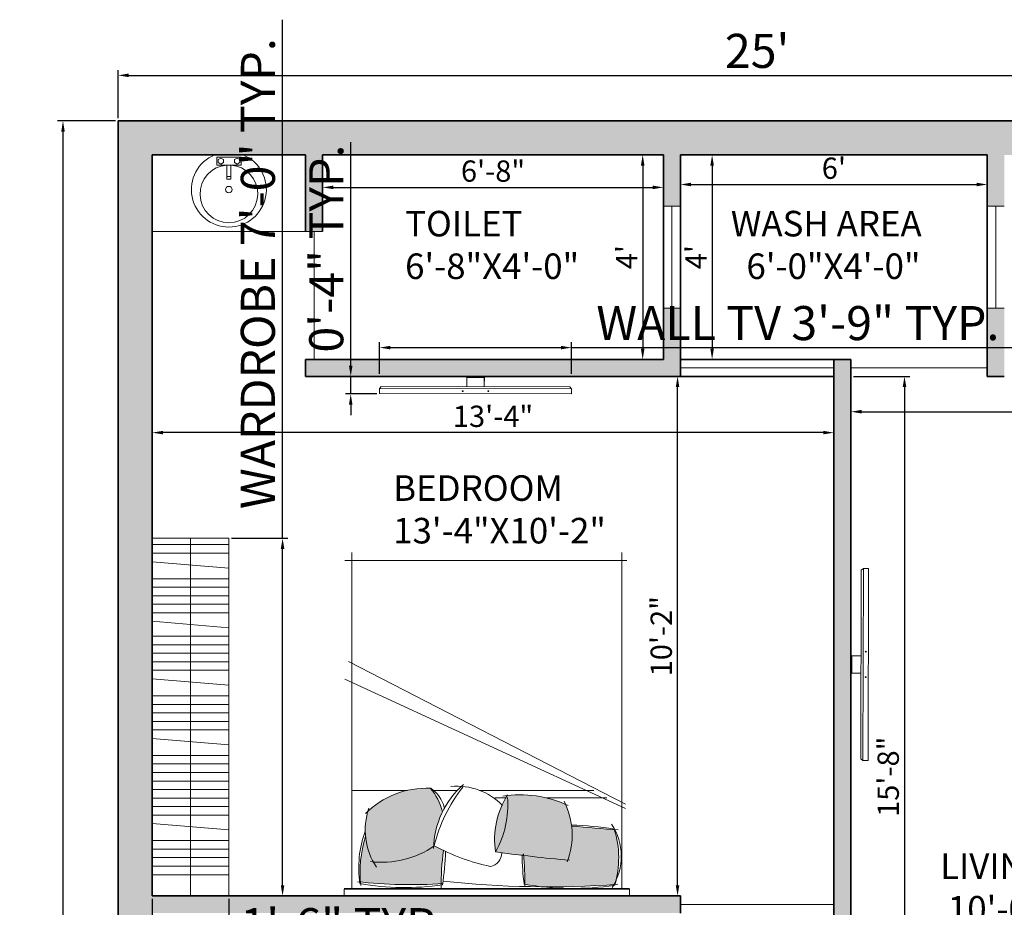
# Model space of a CAD drawing. Units: inches. Extents: x 3259 to 4981, y 1402 to 2026.
# Tile 3 of 11: x 3278 to 3509, y 1722 to 1931. Entities that reach past the tile are written whole.
import ezdxf

# ---------------------------------------------------------------- set-up
doc = ezdxf.new("R2010")
doc.units = ezdxf.units.IN
for name, color, linetype, lineweight in [('0.10', 252, 'Continuous', 9), ('A-ANNO-DIMS', 2, 'Continuous', 13), ('A-AREA-IDEN', 7, 'Continuous', 18), ('A-DOOR', 3, 'Continuous', 18), ('A-EQPM', 8, 'Continuous', 18), ('A-FLOR-CASE', 8, 'Continuous', 18), ('A-FLOR-FIXT', 9, 'Continuous', 18), ('A-FURN', 8, 'Continuous', 13), ('A-GLAZ', 4, 'Continuous', 18), ('A-WALL', 7, 'Continuous', 35), ('A-WALL-PATT', 252, 'Continuous', 13)]:
    doc.layers.add(name, color=color, linetype=linetype, lineweight=lineweight)
doc.layers.add('A-FURN-PATT', color=116, linetype='Continuous', lineweight=13, true_color=0x136734)
doc.styles.get("Standard").update_dxf_attribs({"font": 'arial.ttf'})
doc.dimstyles.new('ISO-25', dxfattribs={"dimtxt": 8, "dimasz": 2.5, "dimexe": 1.25, "dimexo": 0.625, "dimtad": 1, "dimdec": 1, "dimlunit": 3, "dimtxsty": 'Standard', "dimcen": 2.5, "dimclrd": 4, "dimclre": 4, "dimclrt": 1, "dimadec": 0, "dimazin": 0, "dimtfac": 1, "dimtdec": 1, "dimtmove": 0, "dimatfit": 3, "dimfxl": 1, "dimarcsym": 0})

# ---------------------------------------------------------------- blocks, each defined once
blk = doc.blocks.new('camita')
at = {"layer": '0.10'}
for p, q in [((-0.85, -0.045), (0.85, -0.045)), ((-0.805, -0.045), (-0.805, -2.0485)), ((0.805, -0.045), (0.805, -2.0485)), ((-0.8271, -0.521), (0.8464, -1.2932)), ((-0.8271, -0.5476), (0.8236, -1.3992)), ((-0.7161, -0.585), (-0.3554, -0.585)), ((-0.1136, -0.585), (-0.0485, -0.585)), ((-0.638, -0.63), (0.0434, -0.63)), ((0.1749, -0.63), (0.3179, -0.63)), ((0.4739, -0.63), (0.805, -0.63)), ((-0.8354, -2), (0.8464, -2))]:
    blk.add_line(p, q, dxfattribs=at)
blk.add_lwpolyline([(-0.85, -0.0405), (0.85, -0.0405), (0.85, 0), (-0.85, 0)], close=True, dxfattribs=at)
for centre, radius, start, end in [((-0.4574, -0.2364), 0.3443, 147.50996, 213.83359), ((-0.3639, -5.8457), 5.7909, 83.80731, 94.12107), ((-0.5104, -1.7232), 1.6781, 80.12554, 98.66187), ((2.3534, -0.0532), 2.5803, 180.10628, 184.38541), ((-1.4396, -0.0609), 1.7117, 352.92911, 0.39592), ((0.4863, -1.6286), 1.5781, 80.16015, 98.05996), ((-0.1997, -0.2266), 0.5864, 163.92635, 197.14087), ((-1.5443, -0.2452), 1.3333, 359.93941, 7.55329), ((1.5815, -0.2893), 1.3353, 170.38021, 178.99138), ((0.4524, -3.0675), 2.9996, 83.90257, 93.67595), ((0.0294, -0.1377), 0.7262, 342.58415, 6.00484), ((0.1326, -0.1696), 0.6307, 339.92303, 8.74334), ((0.3203, -0.3944), 0.4043, 341.45245, 33.45121), ((-0.0543, -0.3633), 0.4542, 159.30257, 206.50263), ((-1.3301, -9.6748), 9.4985, 82.27078, 84.93989), ((-0.007, -0.258), 0.0828, 100.01798, 179.73597), ((-0.2931, -1.4378), 1.2903, 61.97485, 77.84351), ((0.6265, -0.7518), 0.5508, 82.96906, 124.67388), ((0.4585, -0.5454), 0.5842, 151.04555, 184.14969), ((-0.5341, -0.3393), 0.4875, 327.26442, 9.0473), ((-0.1986, -0.2742), 0.5159, 310.73945, 359.05759), ((-0.5673, -0.0868), 0.9057, 321.69527, 346.46261), ((-1.8672, -14.986), 14.6323, 84.65974, 85.75157), ((-0.4598, 1.4861), 1.9092, 260.95299, 268.65169), ((0.5707, -0.4317), 0.3145, 192.93877, 221.96363), ((0.3612, -0.133), 0.5096, 267.25889, 315.29965), ((-0.2002, 0.064), 0.6673, 244.78094, 279.06058), ((0.179, -0.272), 0.3828, 224.52836, 275.22287), ((0.4384, -0.4834), 0.1898, 193.68485, 236.70352)]:
    blk.add_arc(centre, radius, start, end, dxfattribs=at)
blk = doc.blocks.new('M_BATH_BASIN_Basin - Oval_P')
at = {"color": 0, "linetype": 'ByBlock', "lineweight": -2}
blk.add_lwpolyline([(0, 89.5, -5.027337), (0, -89.5)], format="xyb", close=True, dxfattribs=at)
blk.add_lwpolyline([(63.2, 12, -30), (63.2, -12, -1.097889)], format="xyb", dxfattribs=at)
for points in [[(13.2, -76.2), (13.2, 76.2), (63.2, 76.2), (63.2, -76.2)], [(19.1, 50.8), (28.7, 67.3), (47.7, 67.3), (57.2, 50.8), (47.7, 34.3), (28.7, 34.3)]]:
    blk.add_lwpolyline(points, close=True, dxfattribs=at)
for points in [[(63.2, 12), (151.6, 12), (151.6, -12), (63.2, -12)], [(134.3, 12), (134.3, -12)], [(28.7, -34.3), (47.7, -34.3), (57.2, -50.8), (47.7, -67.3), (28.7, -67.3), (19.1, -50.8), (28.7, -34.3)]]:
    blk.add_lwpolyline(points, dxfattribs=at)
blk.add_circle((216.2, 0), 20.1, dxfattribs=at)
at = {"layer": 'Defpoints'}
for p in [(0, 234), (0, -234)]:
    blk.add_point(p, dxfattribs=at)
blk = doc.blocks.new('*D21')
at = {"layer": 'A-ANNO-DIMS', "color": 0, "lineweight": -2, "transparency": 16777216}
for p, q in [((3301.16, 1907.74), (3301.16, 1919.06)), ((3601.16, 1907.74), (3601.16, 1919.06)), ((3303.66, 1917.81), (3598.66, 1917.81))]:
    blk.add_line(p, q, dxfattribs=at)
at = {"layer": 'A-ANNO-DIMS', "color": 0, "transparency": 16777216}
for points in [[(3303.66, 1918.23), (3303.66, 1917.39), (3301.16, 1917.81)], [(3598.66, 1918.23), (3598.66, 1917.39), (3601.16, 1917.81)]]:
    blk.add_solid(points, dxfattribs=at)
at = {"layer": 'Defpoints', "color": 0, "transparency": 16777216}
for p in [(3601.16, 1917.81), (3301.16, 1907.12), (3601.16, 1907.12)]:
    blk.add_point(p, dxfattribs=at)
at = {"layer": 'A-ANNO-DIMS', "color": 0, "transparency": 16777216, "insert": (3451.16, 1922.52), "char_height": 8, "attachment_point": 5}
blk.add_mtext("25'", dxfattribs=at)
blk = doc.blocks.new('*D22')
at = {"layer": 'A-ANNO-DIMS', "color": 0, "lineweight": -2, "transparency": 16777216}
for p, q in [((3300.54, 1907.12), (3286.97, 1907.12)), ((3288.22, 1904.62), (3288.22, 1477.62)), ((3300.54, 1475.12), (3286.97, 1475.12))]:
    blk.add_line(p, q, dxfattribs=at)
at = {"layer": 'A-ANNO-DIMS', "color": 0, "transparency": 16777216}
for points in [[(3287.81, 1904.62), (3288.64, 1904.62), (3288.22, 1907.12)], [(3287.81, 1477.62), (3288.64, 1477.62), (3288.22, 1475.12)]]:
    blk.add_solid(points, dxfattribs=at)
at = {"layer": 'Defpoints', "color": 0, "transparency": 16777216}
for p in [(3301.16, 1907.12), (3288.22, 1475.12), (3301.16, 1475.12)]:
    blk.add_point(p, dxfattribs=at)
at = {"layer": 'A-ANNO-DIMS', "color": 0, "transparency": 16777216, "insert": (3283.51, 1691.12), "char_height": 8, "attachment_point": 5, "rotation": 90}
blk.add_mtext("36'", dxfattribs=at)
blk = doc.blocks.new('*D23')
at = {"layer": 'A-ANNO-DIMS', "color": 0, "lineweight": -2, "transparency": 16777216}
for p, q in [((3309.16, 1846.49), (3309.16, 1832.67)), ((3469.16, 1846.49), (3469.16, 1832.67)), ((3466.66, 1833.92), (3311.66, 1833.92))]:
    blk.add_line(p, q, dxfattribs=at)
at = {"layer": 'A-ANNO-DIMS', "color": 0, "transparency": 16777216}
for points in [[(3311.66, 1834.34), (3311.66, 1833.51), (3309.16, 1833.92)], [(3466.66, 1834.34), (3466.66, 1833.51), (3469.16, 1833.92)]]:
    blk.add_solid(points, dxfattribs=at)
at = {"layer": 'Defpoints', "color": 0, "transparency": 16777216}
for p in [(3309.16, 1847.12), (3469.16, 1847.12), (3309.16, 1833.92)]:
    blk.add_point(p, dxfattribs=at)
at = {"layer": 'A-ANNO-DIMS', "color": 0, "transparency": 16777216, "insert": (3389.16, 1837.1), "char_height": 5, "attachment_point": 5}
blk.add_mtext('13\'-4"', dxfattribs=at)
blk = doc.blocks.new('*D24')
at = {"layer": 'A-ANNO-DIMS', "color": 0, "lineweight": -2, "transparency": 16777216}
for p, q in [((3432.54, 1847.12), (3431.22, 1847.12)), ((3432.47, 1727.62), (3432.47, 1844.62)), ((3432.54, 1725.12), (3431.22, 1725.12))]:
    blk.add_line(p, q, dxfattribs=at)
at = {"layer": 'A-ANNO-DIMS', "color": 0, "transparency": 16777216}
for points in [[(3432.05, 1844.62), (3432.89, 1844.62), (3432.47, 1847.12)], [(3432.05, 1727.62), (3432.89, 1727.62), (3432.47, 1725.12)]]:
    blk.add_solid(points, dxfattribs=at)
at = {"layer": 'Defpoints', "color": 0, "transparency": 16777216}
for p in [(3432.47, 1847.12), (3433.16, 1847.12), (3433.16, 1725.12)]:
    blk.add_point(p, dxfattribs=at)
at = {"layer": 'A-ANNO-DIMS', "color": 0, "transparency": 16777216, "insert": (3429.29, 1786.12), "char_height": 5, "attachment_point": 5, "rotation": 90}
blk.add_mtext('10\'-2"', dxfattribs=at)
blk = doc.blocks.new('*D25')
at = {"layer": 'A-ANNO-DIMS', "color": 0, "lineweight": -2, "transparency": 16777216}
for p, q in [((3593.16, 1846.49), (3593.16, 1837.58)), ((3473.16, 1843.37), (3473.16, 1837.58)), ((3475.66, 1838.83), (3590.66, 1838.83))]:
    blk.add_line(p, q, dxfattribs=at)
at = {"layer": 'A-ANNO-DIMS', "color": 0, "transparency": 16777216}
for points in [[(3475.66, 1839.25), (3475.66, 1838.42), (3473.16, 1838.83)], [(3590.66, 1839.25), (3590.66, 1838.42), (3593.16, 1838.83)]]:
    blk.add_solid(points, dxfattribs=at)
at = {"layer": 'Defpoints', "color": 0, "transparency": 16777216}
for p in [(3593.16, 1847.12), (3473.16, 1844), (3593.16, 1838.83)]:
    blk.add_point(p, dxfattribs=at)
at = {"layer": 'A-ANNO-DIMS', "color": 0, "transparency": 16777216, "insert": (3533.16, 1842.01), "char_height": 5, "attachment_point": 5}
blk.add_mtext("10'", dxfattribs=at)
blk = doc.blocks.new('*D26')
at = {"layer": 'A-ANNO-DIMS', "color": 0, "lineweight": -2, "transparency": 16777216}
for p, q in [((3473.79, 1847.12), (3486.99, 1847.12)), ((3485.74, 1844.62), (3485.74, 1661.62)), ((3473.79, 1659.12), (3486.99, 1659.12))]:
    blk.add_line(p, q, dxfattribs=at)
at = {"layer": 'A-ANNO-DIMS', "color": 0, "transparency": 16777216}
for points in [[(3485.32, 1844.62), (3486.16, 1844.62), (3485.74, 1847.12)], [(3485.32, 1661.62), (3486.16, 1661.62), (3485.74, 1659.12)]]:
    blk.add_solid(points, dxfattribs=at)
at = {"layer": 'Defpoints', "color": 0, "transparency": 16777216}
for p in [(3473.16, 1847.12), (3473.16, 1659.12), (3485.74, 1659.12)]:
    blk.add_point(p, dxfattribs=at)
at = {"layer": 'A-ANNO-DIMS', "color": 0, "transparency": 16777216, "insert": (3482.56, 1753.12), "char_height": 5, "attachment_point": 5, "rotation": 90}
blk.add_mtext('15\'-8"', dxfattribs=at)
blk = doc.blocks.new('*D35')
at = {"layer": 'A-ANNO-DIMS', "color": 0, "lineweight": -2, "transparency": 16777216}
for p, q in [((3349.16, 1898.49), (3349.16, 1890.25)), ((3429.16, 1898.49), (3429.16, 1890.25)), ((3351.66, 1891.5), (3426.66, 1891.5))]:
    blk.add_line(p, q, dxfattribs=at)
at = {"layer": 'A-ANNO-DIMS', "color": 0, "transparency": 16777216}
for points in [[(3351.66, 1891.92), (3351.66, 1891.09), (3349.16, 1891.5)], [(3426.66, 1891.92), (3426.66, 1891.09), (3429.16, 1891.5)]]:
    blk.add_solid(points, dxfattribs=at)
at = {"layer": 'Defpoints', "color": 0, "transparency": 16777216}
for p in [(3349.16, 1899.12), (3429.16, 1899.12), (3429.16, 1891.5)]:
    blk.add_point(p, dxfattribs=at)
at = {"layer": 'A-ANNO-DIMS', "color": 0, "transparency": 16777216, "insert": (3389.16, 1894.68), "char_height": 5, "attachment_point": 5}
blk.add_mtext('6\'-8"', dxfattribs=at)
blk = doc.blocks.new('*D36')
at = {"layer": 'A-ANNO-DIMS', "color": 0, "lineweight": -2, "transparency": 16777216}
for p, q in [((3428.54, 1899.12), (3423.04, 1899.12)), ((3424.29, 1896.62), (3424.29, 1853.62)), ((3428.54, 1851.12), (3423.04, 1851.12))]:
    blk.add_line(p, q, dxfattribs=at)
at = {"layer": 'A-ANNO-DIMS', "color": 0, "transparency": 16777216}
for points in [[(3423.87, 1896.62), (3424.71, 1896.62), (3424.29, 1899.12)], [(3423.87, 1853.62), (3424.71, 1853.62), (3424.29, 1851.12)]]:
    blk.add_solid(points, dxfattribs=at)
at = {"layer": 'Defpoints', "color": 0, "transparency": 16777216}
for p in [(3429.16, 1899.12), (3424.29, 1851.12), (3429.16, 1851.12)]:
    blk.add_point(p, dxfattribs=at)
at = {"layer": 'A-ANNO-DIMS', "color": 0, "transparency": 16777216, "insert": (3421.17, 1875.12), "char_height": 5, "attachment_point": 5, "rotation": 90}
blk.add_mtext("4'", dxfattribs=at)
blk = doc.blocks.new('*D37')
at = {"layer": 'A-ANNO-DIMS', "color": 0, "lineweight": -2, "transparency": 16777216}
for p, q in [((3433.16, 1898.49), (3433.16, 1890.93)), ((3505.16, 1898.49), (3505.16, 1890.93)), ((3435.66, 1892.18), (3502.66, 1892.18))]:
    blk.add_line(p, q, dxfattribs=at)
at = {"layer": 'A-ANNO-DIMS', "color": 0, "transparency": 16777216}
for points in [[(3435.66, 1892.6), (3435.66, 1891.76), (3433.16, 1892.18)], [(3502.66, 1892.6), (3502.66, 1891.76), (3505.16, 1892.18)]]:
    blk.add_solid(points, dxfattribs=at)
at = {"layer": 'Defpoints', "color": 0, "transparency": 16777216}
for p in [(3433.16, 1899.12), (3505.16, 1899.12), (3505.16, 1892.18)]:
    blk.add_point(p, dxfattribs=at)
at = {"layer": 'A-ANNO-DIMS', "color": 0, "transparency": 16777216, "insert": (3469.16, 1895.36), "char_height": 5, "attachment_point": 5}
blk.add_mtext("6'", dxfattribs=at)
blk = doc.blocks.new('*D38')
at = {"layer": 'A-ANNO-DIMS', "color": 0, "lineweight": -2, "transparency": 16777216}
for p, q in [((3433.79, 1899.12), (3441.83, 1899.12)), ((3440.58, 1896.62), (3440.58, 1853.62)), ((3433.79, 1851.12), (3441.83, 1851.12))]:
    blk.add_line(p, q, dxfattribs=at)
at = {"layer": 'A-ANNO-DIMS', "color": 0, "transparency": 16777216}
for points in [[(3440.16, 1896.62), (3441, 1896.62), (3440.58, 1899.12)], [(3440.16, 1853.62), (3441, 1853.62), (3440.58, 1851.12)]]:
    blk.add_solid(points, dxfattribs=at)
at = {"layer": 'Defpoints', "color": 0, "transparency": 16777216}
for p in [(3433.16, 1899.12), (3433.16, 1851.12), (3440.58, 1851.12)]:
    blk.add_point(p, dxfattribs=at)
at = {"layer": 'A-ANNO-DIMS', "color": 0, "transparency": 16777216, "insert": (3437.45, 1875.12), "char_height": 5, "attachment_point": 5, "rotation": 90}
blk.add_mtext("4'", dxfattribs=at)
blk = doc.blocks.new('WARDROBE-84IN')
for p, q in [((0, 84), (18, 84)), ((9, 0), (9, 84)), ((18, 0), (18, 84)), ((18, 82.5), (0, 82.5)), ((18, 80.5), (0, 80.5)), ((18, 77), (0, 78.5)), ((18, 74.5), (0, 74.5)), ((18, 72.5), (0, 72.5)), ((18, 70.5), (0, 70.5)), ((18, 68.5), (0, 68.5)), ((18, 66.5), (0, 66.5)), ((18, 63), (0, 64.5)), ((18, 61), (0, 61)), ((18, 59), (0, 59)), ((18, 57), (0, 57)), ((18, 55), (0, 55)), ((18, 53), (0, 53)), ((18, 49.5), (0, 51)), ((18, 47), (0, 47)), ((18, 45), (0, 45)), ((18, 43), (0, 43)), ((18, 41), (0, 41)), ((18, 39), (0, 39)), ((18, 35.5), (0, 37)), ((18, 33), (0, 33)), ((18, 31), (0, 31)), ((18, 29), (0, 29)), ((18, 27), (0, 27)), ((18, 25), (0, 25)), ((18, 23), (0, 23)), ((18, 21), (0, 21)), ((18, 19), (0, 19)), ((18, 15.5), (0, 17)), ((18, 13), (0, 13)), ((18, 11), (0, 11)), ((18, 9), (0, 9)), ((18, 7), (0, 7)), ((18, 5), (0, 5))]:
    blk.add_line(p, q)
blk = doc.blocks.new('TV-WALL-MOUNT')
for p, q in [((20.48, 4.12), (20.47, 1.73)), ((20.48, 4.12), (20.52, 4.12)), ((20.52, 4.12), (20.52, 1.73)), ((20.52, 3.88), (24.55, 3.88)), ((24.55, 4.12), (24.55, 1.72)), ((24.55, 4.12), (24.6, 4.12)), ((24.6, 4.12), (24.59, 1.72)), ((0, 1.29), (0.41, 1.77)), ((0.41, 1.77), (44.66, 1.68)), ((45.06, 1.2), (44.66, 1.68))]:
    blk.add_line(p, q)
blk.add_lwpolyline([(0, 0.09), (45.06, 0), (45.06, 1.2), (0, 1.29), (0, 0.09)])
for centre in [(19.53, 0.65), (25.53, 0.64)]:
    blk.add_circle(centre, 0.0959)
blk = doc.blocks.new('VENT-24x4')
for p, q in [((0, 24), (4, 24)), ((2, 24), (2, 0)), ((0, 0), (4, 0))]:
    blk.add_line(p, q)
blk = doc.blocks.new('*D164')
at = {"layer": 'A-ANNO-DIMS', "color": 4, "lineweight": -2, "transparency": 16777216}
for p, q in [((3339.76, 1809.12), (3339.76, 1930.88)), ((3327.79, 1809.12), (3341.01, 1809.12)), ((3339.76, 1727.62), (3339.76, 1806.62)), ((3327.79, 1725.12), (3341.01, 1725.12))]:
    blk.add_line(p, q, dxfattribs=at)
at = {"layer": 'A-ANNO-DIMS', "color": 4, "transparency": 16777216}
for points in [[(3339.35, 1806.62), (3340.18, 1806.62), (3339.76, 1809.12)], [(3339.35, 1727.62), (3340.18, 1727.62), (3339.76, 1725.12)]]:
    blk.add_solid(points, dxfattribs=at)
at = {"layer": 'Defpoints', "color": 0, "transparency": 16777216}
for p in [(3327.16, 1809.12), (3339.76, 1809.12), (3327.16, 1725.12)]:
    blk.add_point(p, dxfattribs=at)
at = {"layer": 'A-ANNO-DIMS', "color": 1, "transparency": 16777216, "insert": (3335, 1871.25), "char_height": 8, "attachment_point": 5, "rotation": 90}
blk.add_mtext('WARDROBE 7\'-0" TYP.', dxfattribs=at)
blk = doc.blocks.new('*D165')
at = {"layer": 'A-ANNO-DIMS', "color": 4, "lineweight": -2, "transparency": 16777216}
for p, q in [((3309.16, 1724.49), (3309.16, 1711.27)), ((3327.16, 1724.49), (3327.16, 1711.27)), ((3311.66, 1712.52), (3324.66, 1712.52)), ((3327.16, 1712.52), (3378.93, 1712.52))]:
    blk.add_line(p, q, dxfattribs=at)
at = {"layer": 'A-ANNO-DIMS', "color": 4, "transparency": 16777216}
for points in [[(3311.66, 1712.93), (3311.66, 1712.1), (3309.16, 1712.52)], [(3324.66, 1712.93), (3324.66, 1712.1), (3327.16, 1712.52)]]:
    blk.add_solid(points, dxfattribs=at)
at = {"layer": 'Defpoints', "color": 0, "transparency": 16777216}
for p in [(3309.16, 1725.12), (3327.16, 1725.12), (3327.16, 1712.52)]:
    blk.add_point(p, dxfattribs=at)
at = {"layer": 'A-ANNO-DIMS', "color": 1, "transparency": 16777216, "insert": (3354.29, 1717.23), "char_height": 8, "attachment_point": 5}
blk.add_mtext('1\'-6" TYP.', dxfattribs=at)
blk = doc.blocks.new('*D168')
at = {"layer": 'A-ANNO-DIMS', "color": 4, "lineweight": -2, "transparency": 16777216}
for p, q in [((3362.52, 1847.75), (3362.52, 1855.13)), ((3365.02, 1853.88), (3405.08, 1853.88)), ((3407.58, 1847.75), (3407.58, 1855.13)), ((3407.58, 1853.88), (3511.34, 1853.88))]:
    blk.add_line(p, q, dxfattribs=at)
at = {"layer": 'A-ANNO-DIMS', "color": 4, "transparency": 16777216}
for points in [[(3365.02, 1854.3), (3365.02, 1853.47), (3362.52, 1853.88)], [(3405.08, 1854.3), (3405.08, 1853.47), (3407.58, 1853.88)]]:
    blk.add_solid(points, dxfattribs=at)
at = {"layer": 'Defpoints', "color": 0, "transparency": 16777216}
for p in [(3407.58, 1853.88), (3362.52, 1847.13), (3407.58, 1847.13)]:
    blk.add_point(p, dxfattribs=at)
at = {"layer": 'A-ANNO-DIMS', "color": 1, "transparency": 16777216, "insert": (3460.71, 1858.6), "char_height": 8, "attachment_point": 5}
blk.add_mtext('WALL TV 3\'-9" TYP.', dxfattribs=at)
blk = doc.blocks.new('*D169')
at = {"layer": 'A-ANNO-DIMS', "color": 4, "lineweight": -2, "transparency": 16777216}
for p, q in [((3355.76, 1849.63), (3355.76, 1902.14)), ((3361.89, 1847.13), (3354.51, 1847.13)), ((3355.76, 1843), (3355.76, 1847.13)), ((3361.89, 1843), (3354.51, 1843)), ((3355.76, 1840.5), (3355.76, 1838))]:
    blk.add_line(p, q, dxfattribs=at)
at = {"layer": 'A-ANNO-DIMS', "color": 4, "transparency": 16777216}
for points in [[(3355.34, 1849.63), (3356.17, 1849.63), (3355.76, 1847.13)], [(3355.34, 1840.5), (3356.17, 1840.5), (3355.76, 1843)]]:
    blk.add_solid(points, dxfattribs=at)
at = {"layer": 'Defpoints', "color": 0, "transparency": 16777216}
for p in [(3355.76, 1847.13), (3362.52, 1847.13), (3362.52, 1843)]:
    blk.add_point(p, dxfattribs=at)
at = {"layer": 'A-ANNO-DIMS', "color": 1, "transparency": 16777216, "insert": (3351.05, 1877.13), "char_height": 8, "attachment_point": 5, "rotation": 90}
blk.add_mtext('0\'-4" TYP.', dxfattribs=at)

msp = doc.modelspace()

# ---------------------------------------------------------------- hatches: boundary and pattern name
at = {"layer": 'A-FURN-PATT'}
h = msp.add_hatch(color=256, dxfattribs=at)
h.dxf.hatch_style = 1
h.paths.add_polyline_path([(3392.47, 1748.69, 0.181694), (3389.77, 1735.46, 0.011408), (3406.73, 1733.55, 0.189536), (3406.2, 1746.63, 0.134508)])
h.paths.add_polyline_path([(3375.22, 1736.79, -0.104045), (3377.29, 1744.89, 0.127326), (3374.43, 1750.4, 0.202559), (3359.77, 1745.01, 0.194952), (3361.05, 1733.12, 0.173835)])
h = msp.add_hatch(color=256, dxfattribs=at)
h.dxf.hatch_style = 1
h.paths.add_polyline_path([(3407.59, 1741.55, -0.113891), (3406.73, 1733.55, -0.006967), (3396.36, 1734.62, -0.016701), (3396.63, 1727.84, 0.015442), (3400.67, 1727.28, 0.01851), (3417.54, 1727.8, 0.020657), (3418.04, 1728.8, 0.131047), (3417.67, 1740.69, -0.004387)])
h.paths.add_polyline_path([(3377.5, 1735.81, -0.011742), (3375.36, 1736.88, -0.175864), (3361.05, 1733.12, -0.098488), (3359.24, 1739.06, 0.094792), (3358.02, 1728.39, 0.040212), (3376.99, 1728, -0.029051)])
at = {"layer": 'A-WALL-PATT'}
h = msp.add_hatch(color=256, dxfattribs=at)
h.dxf.hatch_style = 1
h.paths.add_polyline_path([(3601.16, 1907.12), (3301.16, 1907.12), (3301.16, 1475.12), (3398.16, 1475.12), (3398.16, 1483.12), (3309.16, 1483.12), (3309.16, 1579.12), (3421.16, 1579.12), (3421.16, 1583.12), (3309.16, 1583.12), (3309.16, 1721.12), (3433.16, 1721.12), (3433.16, 1725.12), (3309.16, 1725.12), (3309.16, 1899.12), (3345.16, 1899.12), (3345.16, 1881.12), (3349.16, 1881.12), (3349.16, 1899.12), (3429.16, 1899.12), (3429.16, 1887.12), (3433.16, 1887.12), (3433.16, 1899.12), (3505.16, 1899.12), (3505.16, 1887.12), (3509.16, 1887.12), (3509.16, 1899.12), (3593.16, 1899.12), (3593.16, 1851.12), (3539.16, 1851.12), (3539.16, 1847.12), (3593.16, 1847.12), (3593.16, 1659.12), (3587.16, 1659.12), (3587.16, 1651.12), (3593.16, 1651.12), (3593.16, 1475.12), (3601.16, 1475.12)])
h.paths.add_polyline_path([(3433.16, 1863.12), (3429.16, 1863.12), (3429.16, 1851.12), (3345.16, 1851.12), (3345.16, 1847.12), (3382.99, 1847.12), (3382.99, 1847.13), (3383.04, 1847.13), (3383.04, 1847.12), (3387.07, 1847.12), (3387.07, 1847.12), (3387.11, 1847.12), (3433.16, 1847.12)], flags=17)
h.paths.add_polyline_path([(3509.16, 1863.12), (3505.16, 1863.12), (3505.16, 1847.12), (3509.16, 1847.12)], flags=17)
h.paths.add_polyline_path([(3473.16, 1851.12), (3469.16, 1851.12), (3469.16, 1715.12), (3473.16, 1715.12), (3473.16, 1777.43), (3473.16, 1777.43), (3473.16, 1777.47), (3473.16, 1777.47), (3473.16, 1781.5), (3473.16, 1781.5), (3473.16, 1781.55)], flags=17)
h.paths.add_polyline_path([(3491.16, 1659.12), (3473.16, 1659.12), (3473.16, 1667.12), (3469.16, 1667.12), (3469.16, 1483.12), (3473.16, 1483.12), (3473.16, 1651.12), (3491.16, 1651.12)], flags=17)
h.paths.add_polyline_path([(3551.16, 1659.12), (3539.16, 1659.12), (3539.16, 1651.12), (3551.16, 1651.12)], flags=17)
h.paths.add_polyline_path([(3473.16, 1483.12), (3458.16, 1483.12), (3458.16, 1475.12), (3473.16, 1475.12)], flags=17)

# ---------------------------------------------------------------- linework, layer by layer
at = {"layer": 'A-DOOR'}
for p, q in [((3347.16, 1881.12), (3347.16, 1851.12)), ((3473.16, 1849.12), (3505.16, 1849.12)), ((3433.16, 1723.12), (3469.16, 1723.12))]:
    msp.add_line(p, q, dxfattribs=at)
at = {"layer": 'A-FLOR-CASE'}
msp.add_line((3309.16, 1881.12), (3349.16, 1881.12), dxfattribs=at)
at = {"layer": 'A-GLAZ'}
msp.add_line((3433.16, 1849.12), (3469.16, 1849.12), dxfattribs=at)
at = {"layer": 'A-WALL'}
for p, q in [((3309.16, 1899.12), (3345.16, 1899.12)), ((3309.16, 1725.12), (3309.16, 1899.12)), ((3345.16, 1899.12), (3345.16, 1881.12)), ((3349.16, 1899.12), (3349.16, 1881.12)), ((3349.16, 1899.12), (3429.16, 1899.12)), ((3429.16, 1899.12), (3429.16, 1851.12)), ((3433.16, 1899.12), (3433.16, 1847.12)), ((3433.16, 1899.12), (3505.16, 1899.12)), ((3505.16, 1899.12), (3505.16, 1847.12)), ((3345.16, 1851.12), (3429.16, 1851.12)), ((3345.16, 1851.12), (3345.16, 1847.12)), ((3433.16, 1851.12), (3473.16, 1851.12)), ((3469.16, 1715.12), (3469.16, 1851.12)), ((3473.16, 1715.12), (3473.16, 1851.12)), ((3345.16, 1847.12), (3469.16, 1847.12)), ((3505.16, 1847.12), (3509.16, 1847.12)), ((3309.16, 1725.12), (3433.16, 1725.12)), ((3433.16, 1721.12), (3433.16, 1725.12))]:
    msp.add_line(p, q, dxfattribs=at)
msp.add_lwpolyline([(3473.16, 1475.12), (3301.16, 1475.12), (3301.16, 1907.12), (3601.16, 1907.12), (3601.16, 1475.12), (3593.16, 1475.12)], dxfattribs=at)

# ---------------------------------------------------------------- block references
at = {"layer": 'A-EQPM'}
msp.add_blockref('TV-WALL-MOUNT', (3362.52, 1843), dxfattribs=at)
at = {"layer": 'A-EQPM', "rotation": 90}
msp.add_blockref('TV-WALL-MOUNT', (3477.28, 1756.95), dxfattribs=at)
at = {"layer": 'A-FLOR-CASE'}
msp.add_blockref('WARDROBE-84IN', (3309.16, 1725.12), dxfattribs=at)
at = {"layer": 'A-FLOR-FIXT', "xscale": -0.0376189459335944, "yscale": 0.0376189459335944, "zscale": 0.0376189459335944, "rotation": 90}
msp.add_blockref('M_BATH_BASIN_Basin - Oval_P', (3327.16, 1899.12), dxfattribs=at)
at = {"layer": 'A-FURN', "xscale": 39.375, "yscale": 39.375, "zscale": 39.375, "rotation": 180}
msp.add_blockref('camita', (3387.7, 1725.12), dxfattribs=at)
at = {"layer": 'A-GLAZ'}
msp.add_blockref('VENT-24x4', (3429.16, 1863.12), dxfattribs=at)
at = {"layer": 'A-GLAZ', "rotation": 180}
msp.add_blockref('VENT-24x4', (3509.16, 1887.12), dxfattribs=at)

# ---------------------------------------------------------------- texts
at = {"layer": 'A-AREA-IDEN', "char_height": 6, "attachment_point": 1}
for s, width, insert in [('TOILET\\P6\'-8"X4\'-0"', 127.3061, (3368.52, 1885.99)), ('WASH AREA\\P  6\'-0"X4\'-0"', 127.3061, (3444.97, 1885.99)), ('BEDROOM\\P13\'-4"X10\'-2"', 86.9528, (3365.72, 1823.9)), ('LIVING ROOM\\P 10\'-0"X15\'-8"', 127.3061, (3494.1, 1735.12))]:
    msp.add_mtext_dynamic_manual_height_columns(s, width=width, gutter_width=12.5, heights=[0], dxfattribs=dict(at, insert=insert))

# ---------------------------------------------------------------- dimensions: what is measured, and where the dimension line sits
at = {"layer": 'A-ANNO-DIMS'}
for base, p1, p2, text, picture, middle in [((3339.76, 1809.12), (3327.16, 1725.12), (3327.16, 1809.12), 'WARDROBE <> TYP.', '*D164', (3335, 1871.25)), ((3355.76, 1847.13), (3362.52, 1843), (3362.52, 1847.13), '<> TYP.', '*D169', (3351.05, 1877.13))]:
    dim = msp.add_linear_dim(base=base, p1=p1, p2=p2, angle=90, text=text, dimstyle='ISO-25', override={"dimdec": 1, "dimlfac": 1, "dimrnd": 0, "dimzin": 1, "dimdsep": 46, "dimlunit": 4, "dimfrac": 2}, dxfattribs=at)
    dim.commit()
    dim.dimension.update_dxf_attribs({"geometry": picture, "text_midpoint": middle})
for base, p1, p2, override, picture, middle in [((3601.16, 1917.81), (3301.16, 1907.12), (3601.16, 1907.12), {"dimclrd": 0, "dimclre": 0, "dimclrt": 0}, '*D21', (3451.16, 1922.52)), ((3429.16, 1891.5), (3349.16, 1899.12), (3429.16, 1899.12), {"dimtxt": 5, "dimclrd": 0, "dimclre": 0, "dimclrt": 0}, '*D35', (3389.16, 1894.68)), ((3505.16, 1892.18), (3433.16, 1899.12), (3505.16, 1899.12), {"dimtxt": 5, "dimclrd": 0, "dimclre": 0, "dimclrt": 0}, '*D37', (3469.16, 1895.36)), ((3309.16, 1833.92), (3469.16, 1847.12), (3309.16, 1847.12), {"dimtxt": 5, "dimclrd": 0, "dimclre": 0, "dimclrt": 0}, '*D23', (3389.16, 1837.1)), ((3593.16, 1838.83), (3473.16, 1844), (3593.16, 1847.12), {"dimtxt": 5, "dimclrd": 0, "dimclre": 0, "dimclrt": 0}, '*D25', (3533.16, 1842.01))]:
    dim = msp.add_linear_dim(base=base, p1=p1, p2=p2, dimstyle='ISO-25', override=override, dxfattribs=at)
    dim.commit()
    dim.dimension.update_dxf_attribs({"geometry": picture, "text_midpoint": middle})
for base, p1, p2, override, picture, middle in [((3288.22, 1475.12), (3301.16, 1907.12), (3301.16, 1475.12), {"dimclrd": 0, "dimclre": 0, "dimclrt": 0}, '*D22', (3283.51, 1691.12)), ((3424.29, 1851.12), (3429.16, 1899.12), (3429.16, 1851.12), {"dimtxt": 5, "dimclrd": 0, "dimclre": 0, "dimclrt": 0}, '*D36', (3421.17, 1875.12)), ((3440.58, 1851.12), (3433.16, 1899.12), (3433.16, 1851.12), {"dimtxt": 5, "dimclrd": 0, "dimclre": 0, "dimclrt": 0}, '*D38', (3437.45, 1875.12)), ((3432.47, 1847.12), (3433.16, 1725.12), (3433.16, 1847.12), {"dimtxt": 5, "dimclrd": 0, "dimclre": 0, "dimclrt": 0}, '*D24', (3429.29, 1786.12)), ((3485.74, 1659.12), (3473.16, 1847.12), (3473.16, 1659.12), {"dimtxt": 5, "dimclrd": 0, "dimclre": 0, "dimclrt": 0}, '*D26', (3482.56, 1753.12))]:
    dim = msp.add_linear_dim(base=base, p1=p1, p2=p2, angle=90, dimstyle='ISO-25', override=override, dxfattribs=at)
    dim.commit()
    dim.dimension.update_dxf_attribs({"geometry": picture, "text_midpoint": middle})
for base, p1, p2, text, picture, middle in [((3407.58, 1853.88), (3362.52, 1847.13), (3407.58, 1847.13), 'WALL TV <> TYP.', '*D168', (3460.71, 1858.6)), ((3327.16, 1712.52), (3309.16, 1725.12), (3327.16, 1725.12), '<> TYP.', '*D165', (3354.29, 1717.23))]:
    dim = msp.add_linear_dim(base=base, p1=p1, p2=p2, text=text, dimstyle='ISO-25', override={"dimdec": 1, "dimlfac": 1, "dimrnd": 0, "dimzin": 1, "dimdsep": 46, "dimlunit": 4, "dimfrac": 2}, dxfattribs=at)
    dim.commit()
    dim.dimension.update_dxf_attribs({"geometry": picture, "text_midpoint": middle})

doc.saveas('drawing.dxf')
